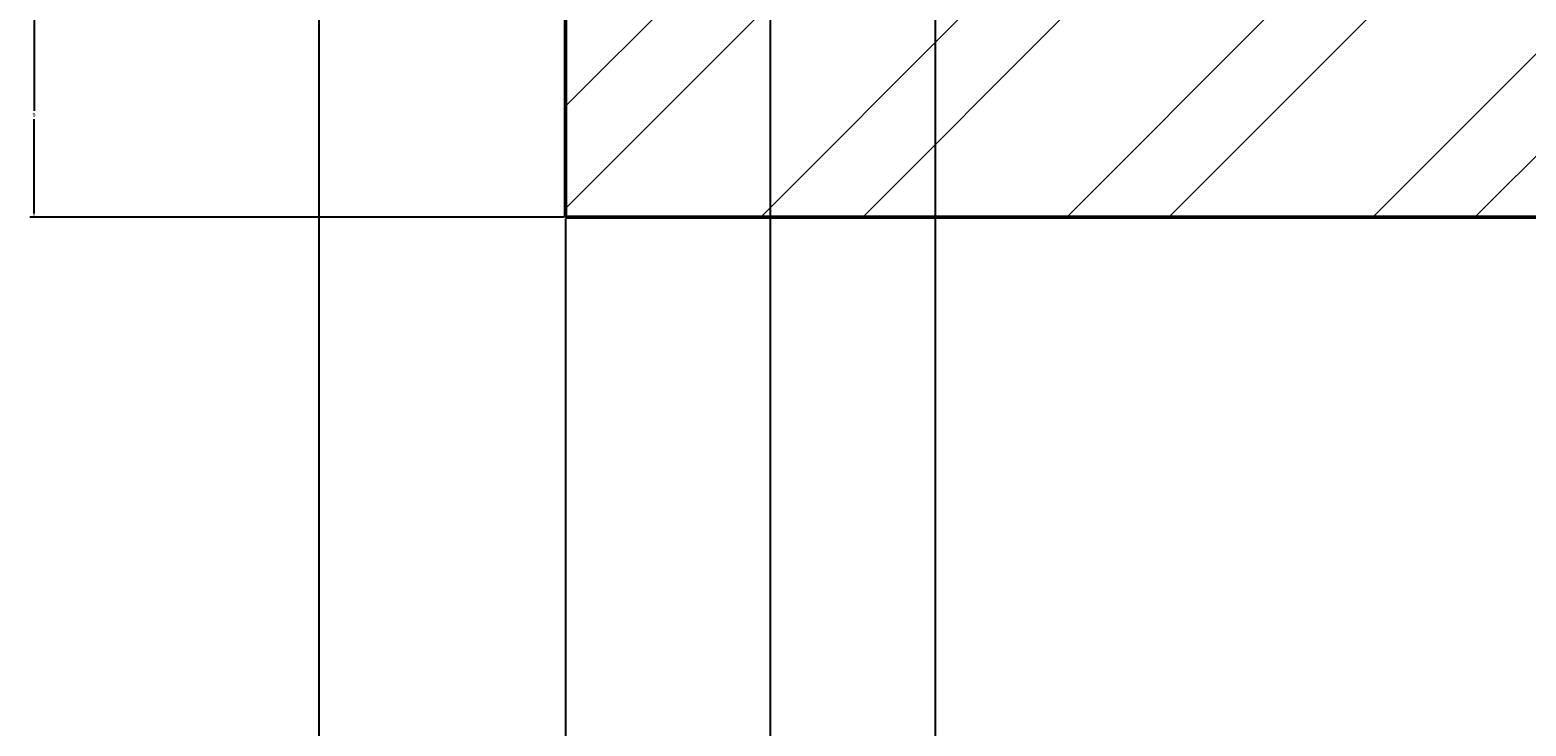
# Model space of a CAD drawing. Units: inches. Extents: x 2812 to 3051, y 1398 to 1659.
# Tile 44 of 65: x 2812 to 2878, y 1528 to 1559. Entities that reach past the tile are written whole.
import ezdxf

# ---------------------------------------------------------------- set-up
doc = ezdxf.new("R2010")
doc.units = ezdxf.units.IN
for name, color, linetype, lineweight in [('A-ANNO-DIMS', 2, 'Continuous', 18), ('S-CONC', 7, 'Continuous', 50), ('S-CONC-PATT', 8, 'Continuous', 18)]:
    doc.layers.add(name, color=color, linetype=linetype, lineweight=lineweight)
doc.styles.get("Standard").update_dxf_attribs({"font": 'arial.ttf'})
doc.dimstyles.get("Standard").update_dxf_attribs({"dimtxt": 0.18, "dimasz": 0.18, "dimexe": 0.18, "dimexo": 0.0625, "dimgap": 0.09, "dimtad": 0, "dimtih": 1, "dimtoh": 1, "dimdec": 4, "dimzin": 0, "dimdsep": 46, "dimtxsty": 'Standard', "dimcen": 0.09, "dimadec": 0, "dimazin": 0, "dimtfac": 1, "dimtdec": 4, "dimtofl": 0, "dimtmove": 0, "dimatfit": 3, "dimfxl": 1, "dimtolj": 1, "dimtzin": 0, "dimarcsym": 0})

# ---------------------------------------------------------------- blocks, each defined once
blk = doc.blocks.new('*D27')
at = {"layer": 'A-ANNO-DIMS', "color": 0, "lineweight": -2, "transparency": 16777216}
for p, q in [((2824.521, 1594.167), (2824.521, 1397.505)), ((2835.385, 1550.757), (2835.385, 1397.505)), ((2824.701, 1397.685), (2829.498, 1397.685)), ((2835.205, 1397.685), (2830.408, 1397.685))]:
    blk.add_line(p, q, dxfattribs=at)
at = {"layer": 'A-ANNO-DIMS', "color": 0, "transparency": 16777216}
for points in [[(2824.701, 1397.715), (2824.701, 1397.655), (2824.521, 1397.685)], [(2835.205, 1397.715), (2835.205, 1397.655), (2835.385, 1397.685)]]:
    blk.add_solid(points, dxfattribs=at)
at = {"layer": 'Defpoints', "color": 0, "transparency": 16777216}
for p in [(2824.521, 1594.23), (2835.385, 1550.82), (2835.385, 1397.685)]:
    blk.add_point(p, dxfattribs=at)
at = {"layer": 'A-ANNO-DIMS', "color": 0, "transparency": 16777216, "insert": (2829.953, 1397.685), "char_height": 0.18, "attachment_point": 5}
blk.add_mtext('\\A1;10.863', dxfattribs=at)
blk = doc.blocks.new('*D28')
at = {"layer": 'A-ANNO-DIMS', "color": 0, "lineweight": -2, "transparency": 16777216}
for p, q in [((2851.646, 1598.667), (2851.646, 1397.505)), ((2844.385, 1559.757), (2844.385, 1397.505)), ((2844.565, 1397.685), (2847.64, 1397.685)), ((2851.466, 1397.685), (2848.391, 1397.685))]:
    blk.add_line(p, q, dxfattribs=at)
at = {"layer": 'A-ANNO-DIMS', "color": 0, "transparency": 16777216}
for points in [[(2844.565, 1397.715), (2844.565, 1397.655), (2844.385, 1397.685)], [(2851.466, 1397.715), (2851.466, 1397.655), (2851.646, 1397.685)]]:
    blk.add_solid(points, dxfattribs=at)
at = {"layer": 'Defpoints', "color": 0, "transparency": 16777216}
for p in [(2851.646, 1598.73), (2844.385, 1559.82), (2851.646, 1397.685)]:
    blk.add_point(p, dxfattribs=at)
at = {"layer": 'A-ANNO-DIMS', "color": 0, "transparency": 16777216, "insert": (2848.016, 1397.685), "char_height": 0.18, "attachment_point": 5}
blk.add_mtext('\\A1;7.261', dxfattribs=at)
blk = doc.blocks.new('*D36')
at = {"layer": 'A-ANNO-DIMS', "color": 0, "lineweight": -2, "transparency": 16777216}
for p, q in [((2844.322, 1559.82), (2811.806, 1559.82)), ((2811.986, 1559.64), (2811.986, 1555.502)), ((2811.986, 1551), (2811.986, 1555.138)), ((2835.322, 1550.82), (2811.806, 1550.82))]:
    blk.add_line(p, q, dxfattribs=at)
at = {"layer": 'A-ANNO-DIMS', "color": 0, "transparency": 16777216}
for points in [[(2811.956, 1559.64), (2812.016, 1559.64), (2811.986, 1559.82)], [(2811.956, 1551), (2812.016, 1551), (2811.986, 1550.82)]]:
    blk.add_solid(points, dxfattribs=at)
at = {"layer": 'Defpoints', "color": 0, "transparency": 16777216}
for p in [(2811.986, 1559.82), (2844.385, 1559.82), (2835.385, 1550.82)]:
    blk.add_point(p, dxfattribs=at)
at = {"layer": 'A-ANNO-DIMS', "color": 0, "transparency": 16777216, "insert": (2811.986, 1555.32), "char_height": 0.18, "attachment_point": 5}
blk.add_mtext('\\A1;9', dxfattribs=at)

msp = doc.modelspace()

# ---------------------------------------------------------------- hatches: boundary and pattern name
at = {"layer": 'S-CONC-PATT'}
h = msp.add_hatch(dxfattribs=at)
h.set_pattern_fill('ANSI32', color=256)
h.paths.add_polyline_path([(3027.3849, 1646.82), (2835.3849, 1646.82), (2835.3849, 1603.2296), (2844.3849, 1603.2296), (2844.3849, 1637.82), (3018.3849, 1637.82), (3018.3849, 1602.5441), (3027.3849, 1602.5441)])
h.paths.add_polyline_path([(2844.3849, 1594.2296), (2835.3849, 1594.2296), (2835.3849, 1550.82), (3027.3849, 1550.82), (3027.3849, 1593.5441), (3018.3849, 1593.5441), (3018.3849, 1559.82), (2844.3849, 1559.82)])
h.paths.add_polyline_path([(2844.3849, 1482.0354), (2835.3849, 1482.0354), (2835.3849, 1463.4959), (2844.3849, 1463.4959)])
h.paths.add_polyline_path([(2844.3849, 1461.4959), (2835.3849, 1461.4959), (2835.3849, 1416.0354), (2844.3849, 1416.0354)])
h.paths.add_polyline_path([(3027.3849, 1482.0354), (3018.3849, 1482.0354), (3018.3849, 1463.2854), (3027.3849, 1463.2854)])
h.paths.add_polyline_path([(3027.3849, 1461.2854), (3018.3849, 1461.2854), (3018.3849, 1416.0354), (3027.3849, 1416.0354)])
h.paths.add_polyline_path([(2961.3849, 1448.4738), (2952.3849, 1448.4738), (2952.3849, 1416.0354), (2961.3849, 1416.0354)])
h.paths.add_polyline_path([(2961.3849, 1462.3026), (2952.3849, 1462.3026), (2952.3849, 1450.4738), (2961.3849, 1450.4738)])
h.paths.add_polyline_path([(2961.3849, 1472.0354), (2952.3849, 1472.0354), (2952.3849, 1462.3026), (2961.3849, 1462.3026)])

# ---------------------------------------------------------------- linework, layer by layer
at = {"layer": 'S-CONC'}
for p, q in [((2835.3849, 1550.82), (2835.3849, 1646.82)), ((3027.3849, 1550.82), (2835.3849, 1550.82))]:
    msp.add_line(p, q, dxfattribs=at)

# ---------------------------------------------------------------- dimensions: what is measured, and where the dimension line sits
at = {"layer": 'A-ANNO-DIMS'}
for base, p1, p2, picture, middle in [((2851.6462, 1397.6854), (2844.3849, 1559.82), (2851.6462, 1598.7296), '*D28', (2848.0156, 1397.6854)), ((2835.384907, 1397.685398), (2824.521409, 1594.229631), (2835.384907, 1550.819971), '*D27', (2829.953158, 1397.685398))]:
    dim = msp.add_linear_dim(base=base, p1=p1, p2=p2, dimstyle='Standard', override={"dimdec": 3, "dimlfac": 1, "dimrnd": 0, "dimzin": 0, "dimdsep": 46, "dimlunit": 2}, dxfattribs=at)
    dim.commit()
    dim.dimension.update_dxf_attribs({"geometry": picture, "text_midpoint": middle})
dim = msp.add_linear_dim(base=(2811.9855, 1559.82), p1=(2835.3849, 1550.82), p2=(2844.3849, 1559.82), angle=90, dimstyle='Standard', override={"dimdec": 0, "dimlfac": 1, "dimrnd": 0, "dimzin": 0, "dimdsep": 46, "dimlunit": 2}, dxfattribs=at)
dim.commit()
dim.dimension.update_dxf_attribs({"geometry": '*D36', "text_midpoint": (2811.9855, 1555.32)})

doc.saveas('drawing.dxf')
